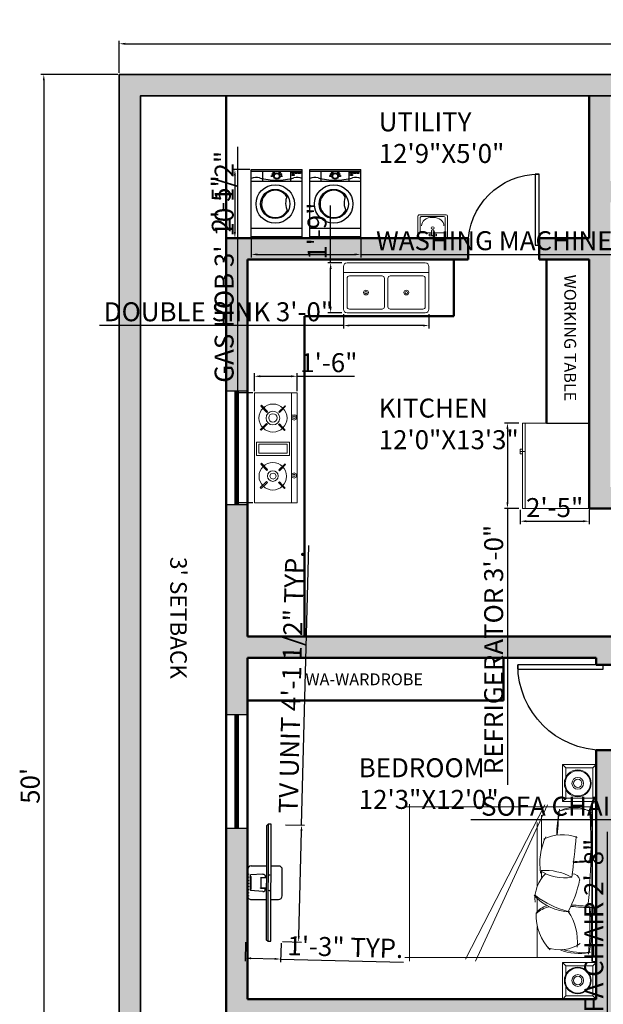
# Model space of a CAD drawing. Units: inches. Extents: x 2442 to 3851, y 589 to 2836.
# Tile 4 of 22: x 2452 to 2698, y 1610 to 2025. Entities that reach past the tile are written whole.
import ezdxf

# ---------------------------------------------------------------- set-up
doc = ezdxf.new("R2010")
doc.units = ezdxf.units.IN
for name, color, linetype, lineweight in [('0.10', 252, 'Continuous', 9), ('0.15', 34, 'Continuous', 15), ('A-ANNO-DIMS', 2, 'Continuous', 18), ('A-ANNO-TEXT', 7, 'Continuous', 18), ('A-AREA-IDEN', 7, 'Continuous', 18), ('A-DOOR', 4, 'Continuous', 25), ('A-EQPM', 9, 'Continuous', 18), ('A-FLOR-FIXT', 8, 'Continuous', 18), ('A-FURN', 8, 'Continuous', 18), ('A-GLAZ', 1, 'Continuous', 25), ('A-WALL', 7, 'Continuous', 50), ('A-WALL-PATT', 8, 'Continuous', 13), ('C-PROP', 7, 'Continuous', 35)]:
    doc.layers.add(name, color=color, linetype=linetype, lineweight=lineweight)
doc.layers.add('window', color=130, linetype='Continuous')
doc.layers.add('Сантехника', color=7, linetype='Continuous')
doc.styles.get("Standard").update_dxf_attribs({"font": 'arial.ttf'})
doc.dimstyles.new('ISO-25', dxfattribs={"dimtxt": 8, "dimasz": 2.5, "dimexe": 1.25, "dimexo": 0.625, "dimtad": 1, "dimlunit": 3, "dimtxsty": 'Standard', "dimcen": 2.5, "dimadec": 0, "dimazin": 0, "dimtfac": 1, "dimtmove": 0, "dimatfit": 3, "dimfxl": 1, "dimarcsym": 0})

# ---------------------------------------------------------------- blocks, each defined once
blk = doc.blocks.new('*U23')
for p, q in [((0, 0), (0, -6)), ((36, 0), (36, -6))]:
    blk.add_line(p, q)
blk.add_lwpolyline([(0, 0), (0, 36), (1.75, 36), (1.75, 0)], close=True)
blk.add_arc((0, 0), 36, 0, 90)
blk = doc.blocks.new('*U24')
for p, q in [((0, 0), (0, -6)), ((30, 0), (30, -6))]:
    blk.add_line(p, q)
blk.add_lwpolyline([(0, 0), (0, 30), (1.75, 30), (1.75, 0)], close=True)
blk.add_arc((0, 0), 30, 0, 90)
blk = doc.blocks.new('Refrigerator-2 door - 36 in top')
for p, q in [((0, -26.999999), (36, -26.999999)), ((11, -27.999999), (11, -28.999999)), ((11, -28.999999), (13, -28.999999)), ((12, -26.999999), (12, -28.999999)), ((13, -28.999999), (13, -27.999999))]:
    blk.add_line(p, q)
blk.add_lwpolyline([(0, -27.999999), (0, 0), (36, 0), (36, -27.999999)], close=True)
blk = doc.blocks.new('camita')
at = {"layer": '0.10'}
for p, q in [((-0.85, -0.045), (0.85, -0.045)), ((-0.805, -0.045), (-0.805, -2.048)), ((0.805, -0.045), (0.805, -2.048)), ((-0.827, -0.521), (0.846, -1.293)), ((-0.827, -0.548), (0.824, -1.399)), ((-0.716, -0.585), (-0.355, -0.585)), ((-0.638, -0.63), (0.043, -0.63)), ((-0.114, -0.585), (-0.049, -0.585)), ((0.175, -0.63), (0.318, -0.63)), ((0.474, -0.63), (0.805, -0.63)), ((-0.835, -2), (0.846, -2))]:
    blk.add_line(p, q, dxfattribs=at)
blk.add_lwpolyline([(-0.85, -0.041), (0.85, -0.041), (0.85, 0), (-0.85, 0)], close=True, dxfattribs=at)
for centre, radius, start, end in [((-0.457, -0.236), 0.344, 147.51, 213.8336), ((-0.2, -0.227), 0.586, 163.9263, 197.1409), ((-0.364, -5.846), 5.791, 83.8073, 94.1211), ((-0.51, -1.723), 1.678, 80.1255, 98.6619), ((2.353, -0.053), 2.58, 180.1063, 184.3854), ((-1.544, -0.245), 1.333, 359.9394, 7.5533), ((1.581, -0.289), 1.335, 170.3802, 178.9914), ((-1.44, -0.061), 1.712, 352.9291, 0.3959), ((0.452, -3.067), 3, 83.9026, 93.6759), ((0.486, -1.629), 1.578, 80.1602, 98.06), ((0.029, -0.138), 0.726, 342.5841, 6.0048), ((0.133, -0.17), 0.631, 339.923, 8.7433), ((-0.054, -0.363), 0.454, 159.3026, 206.5026), ((-0.007, -0.258), 0.0828, 100.018, 179.736), ((-0.293, -1.438), 1.29, 61.9749, 77.8435), ((0.627, -0.752), 0.551, 82.9691, 124.6739), ((0.32, -0.394), 0.404, 341.4524, 33.4512), ((-1.33, -9.675), 9.499, 82.2708, 84.9399), ((0.458, -0.545), 0.584, 151.0456, 184.1497), ((-0.534, -0.339), 0.487, 327.2644, 9.0473), ((-0.199, -0.274), 0.516, 310.7395, 359.0576), ((-0.567, -0.087), 0.906, 321.6953, 346.4626), ((-1.867, -14.986), 14.632, 84.6597, 85.7516), ((-0.46, 1.486), 1.909, 260.953, 268.6517), ((0.571, -0.432), 0.315, 192.9388, 221.9636), ((0.361, -0.133), 0.51, 267.2589, 315.2997), ((-0.2, 0.064), 0.667, 244.7809, 279.0606), ((0.179, -0.272), 0.383, 224.5284, 275.2229), ((0.438, -0.483), 0.19, 193.6849, 236.7035)]:
    blk.add_arc(centre, radius, start, end, dxfattribs=at)
blk = doc.blocks.new('VELADOR')
at = {"layer": '0.15'}
for p, q in [((-0.248, 0), (-0.203, -0.045)), ((0.248, 0), (0.202, -0.045)), ((-0.203, -0.405), (-0.248, -0.45)), ((0.248, -0.45), (0.202, -0.405))]:
    blk.add_line(p, q, dxfattribs=at)
blk.add_lwpolyline([(-0.248, 0), (-0.248, -0.45), (0.248, -0.45), (0.248, 0)], close=True, dxfattribs=at)
blk.add_lwpolyline([(0.092, -0.405), (0.202, -0.405), (0.202, -0.045), (-0.203, -0.045), (-0.203, -0.405), (-0.082, -0.405)], dxfattribs=at)
for radius in [0.18, 0.169, 0.0788, 0.0563]:
    blk.add_circle((0.005, -0.247), radius, dxfattribs=at)
blk = doc.blocks.new('Sink-double - 36 in top')
for p, q in [((-18, -4), (18, -4)), ((-0.75, -18.5), (-0.75, -6.5)), ((0.75, -6.5), (0.75, -18.5))]:
    blk.add_line(p, q)
for points in [[(-16.5, 0), (16.5, 0)], [(-18, -19.5), (-18, -1.5)], [(18, -1.5), (18, -19.5)], [(-16.5, -18.5), (-16.5, -6.5)], [(-15.5, -5.5), (-1.75, -5.5)], [(1.75, -5.5), (15.5, -5.5)], [(16.5, -6.5), (16.5, -18.5)], [(-1.75, -19.5), (-15.5, -19.5)], [(15.5, -19.5), (1.75, -19.5)], [(16.5, -21), (-16.5, -21)]]:
    blk.add_lwpolyline(points)
for centre, radius in [((-8.5, -12.5), 1), ((-8.5, -12.5), 0.5), ((8.5, -12.5), 1), ((8.5, -12.5), 0.5)]:
    blk.add_circle(centre, radius)
for centre, radius, start, end in [((-16.5, -1.5), 1.5, 90, 180), ((16.5, -1.5), 1.5, 0, 90), ((-15.5, -6.5), 1, 90, 180), ((-1.75, -6.5), 1, 0, 90), ((1.75, -6.5), 1, 90, 180), ((15.5, -6.5), 1, 0, 90), ((-16.5, -19.5), 1.5, 180, 270), ((-15.5, -18.5), 1, 180, 270), ((-1.75, -18.5), 1, 270, 0), ((1.75, -18.5), 1, 180, 270), ((15.5, -18.5), 1, 270, 0), ((16.5, -19.5), 1.5, 270, 0)]:
    blk.add_arc(centre, radius, start, end)
blk = doc.blocks.new('gas 1')
for points in [[(35.93, -1.87), (35.93, 0), (0, 0), (0, -1.87)], [(8.12, -0.94), (8.44, -1.56), (8.91, -1.87), (9.53, -1.56), (9.84, -0.94), (9.53, -0.31), (8.91, -0.16), (8.44, -0.31)], [(8.59, -0.94), (8.75, -1.25), (8.91, -1.41), (9.22, -1.25), (9.37, -0.94), (9.22, -0.78), (8.91, -0.62), (8.75, -0.78)], [(19.84, -13.28), (15.47, -13.28), (15.47, -2.5), (19.84, -2.5)], [(27.03, -0.94), (27.34, -1.56), (27.97, -1.87), (28.59, -1.56), (28.75, -0.94), (28.59, -0.31), (27.97, -0.16), (27.34, -0.31)], [(27.5, -0.94), (27.65, -1.25), (27.97, -1.41), (28.28, -1.25), (28.28, -0.94), (28.28, -0.62), (27.97, -0.62), (27.65, -0.62)], [(4.84, -3.91), (4.69, -4.06), (6.72, -6.09), (6.87, -5.78)], [(12.81, -3.91), (12.5, -3.75), (10.47, -5.78), (10.78, -5.94)], [(19.22, -12.5), (16.25, -12.5), (16.25, -3.28), (19.22, -3.28)], [(23.75, -3.91), (23.59, -4.06), (25.62, -6.09), (25.78, -5.78)], [(31.71, -3.91), (31.56, -3.75), (29.53, -5.78), (29.68, -5.94)], [(7.81, -7.81), (8.12, -8.59), (8.75, -8.91), (9.53, -8.59), (9.69, -7.81), (9.53, -7.19), (8.75, -6.87), (8.12, -7.19)], [(7.03, -10), (6.72, -9.69), (4.69, -11.72), (5, -12.03)], [(12.97, -11.56), (10.94, -9.69), (10.62, -9.84), (12.65, -11.87)], [(23.75, -11.72), (23.9, -12.03), (25.93, -10), (25.78, -9.69)], [(31.87, -11.56), (29.84, -9.69), (29.53, -9.84), (31.56, -11.87)]]:
    blk.add_lwpolyline(points, close=True)
blk.add_lwpolyline([(35.93, -1.87), (35.93, -13.9), (0, -13.9), (0, -1.87)])
for centre, radius in [((8.7, -7.92), 4.48), ((8.77, -7.89), 1.74), ((27.7, -7.86), 4.58), ((27.69, -7.89), 2.22), ((27.76, -7.89), 1.35)]:
    blk.add_circle(centre, radius)
blk = doc.blocks.new('TV')
at = {"color": 0}
for p, q in [((3967.27, 1784.85), (3967.05, 1784.65)), ((3967.76, 1763.68), (3967.54, 1763.86))]:
    blk.add_line(p, q, dxfattribs=at)
at = {"layer": 'window'}
for p, q in [((3967.54, 1763.86), (3967.05, 1784.65)), ((3964.41, 1777.23), (3967.22, 1777.3)), ((3968.01, 1777.32), (3969.36, 1777.35)), ((3966.53, 1775.82), (3964.33, 1775.61)), ((3964.34, 1775.34), (3964.45, 1775.34)), ((3964.34, 1775.31), (3964.43, 1775.32)), ((3966.14, 1775.2), (3967.01, 1775.22)), ((3966.14, 1775.18), (3967.27, 1775.2)), ((3966.14, 1775.18), (3966.14, 1775.2)), ((3966.3, 1773.29), (3966.26, 1775.18)), ((3966.19, 1773.28), (3967.31, 1773.31)), ((3966.19, 1773.26), (3967.05, 1773.28)), ((3966.19, 1773.26), (3966.19, 1773.28)), ((3964.39, 1773.06), (3964.48, 1773.06)), ((3964.39, 1773.04), (3964.5, 1773.04)), ((3966.61, 1772.66), (3964.4, 1772.77)), ((3964.55, 1771.15), (3967.36, 1771.22)), ((3968.15, 1771.24), (3969.5, 1771.27))]:
    blk.add_line(p, q, dxfattribs=at)
for points in [[(3968.33, 1763.69), (3967.83, 1784.86), (3967.27, 1784.85), (3967.76, 1763.68), (3968.33, 1763.69)], [(3963.86, 1771.81), (3963.75, 1776.54)], [(3964.4, 1772.77), (3964.33, 1775.61)], [(3964.48, 1773.06), (3964.43, 1775.32)], [(3964.5, 1773.04), (3964.45, 1775.34)], [(3970.16, 1771.96), (3970.05, 1776.69)]]:
    blk.add_lwpolyline(points, dxfattribs=at)
for points in [[(3966.53, 1775.82, -0.263666), (3966.93, 1775.69), (3967, 1775.57), (3967.01, 1775.22)], [(3966.61, 1772.66, 0.263666), (3967, 1772.81), (3967.06, 1772.93), (3967.05, 1773.28)]]:
    blk.add_lwpolyline(points, format="xyb", dxfattribs=at)
for centre, radius in [((3963.91, 1775.73), 0.0679), ((3963.93, 1775.17), 0.0679), ((3967.77, 1775.68), 0.0451), ((3963.94, 1774.6), 0.0679), ((3963.95, 1774.04), 0.0679), ((3963.97, 1773.48), 0.0679), ((3963.98, 1772.92), 0.0679), ((3963.99, 1772.35), 0.0679), ((3964.01, 1771.79), 0.0679), ((3967.83, 1772.86), 0.0451)]:
    blk.add_circle(centre, radius, dxfattribs=at)
for centre, start, end in [((3964.42, 1776.56), 91.3414, 181.3414), ((3969.38, 1776.67), 1.3414, 91.3414), ((3964.53, 1771.83), 181.3414, 271.3414), ((3969.49, 1771.94), 271.3414, 1.3414)]:
    blk.add_arc(centre, 0.676, start, end, dxfattribs=at)
blk = doc.blocks.new('wash')
at = {"layer": 'Сантехника'}
for p, q in [((4817.13, 2840.92), (4788.24, 2840.92)), ((4788.24, 2819.46), (4788.24, 2840.92)), ((4788.93, 2819.46), (4788.93, 2840.92)), ((4793.08, 2819.46), (4793.08, 2840.92)), ((4812.98, 2819.46), (4812.98, 2840.92)), ((4816.44, 2819.46), (4816.44, 2840.92)), ((4817.13, 2819.46), (4817.13, 2840.92)), ((4793.08, 2836.07), (4788.93, 2836.07)), ((4793.08, 2824.31), (4788.93, 2824.31)), ((4817.13, 2819.46), (4788.24, 2819.46)), ((4817.13, 2816.27), (4788.24, 2816.27)), ((4788.24, 2794.82), (4788.24, 2816.27)), ((4788.93, 2794.82), (4788.93, 2816.27)), ((4793.08, 2794.82), (4793.08, 2816.27)), ((4812.98, 2794.82), (4812.98, 2816.27)), ((4816.44, 2794.82), (4816.44, 2816.27)), ((4817.13, 2794.82), (4817.13, 2816.27)), ((4793.08, 2811.43), (4788.93, 2811.43)), ((4793.08, 2799.66), (4788.93, 2799.66)), ((4817.13, 2794.82), (4788.24, 2794.82))]:
    blk.add_line(p, q, dxfattribs=at)
for points in [[(4789.4, 2839.27), (4789.4, 2840.17), (4789.9, 2840.17), (4789.9, 2839.27)], [(4789.4, 2837.95), (4789.4, 2838.85), (4789.9, 2838.85), (4789.9, 2837.95)], [(4789.4, 2836.64), (4789.4, 2837.53), (4789.9, 2837.53), (4789.9, 2836.64)], [(4790.27, 2836.64), (4790.27, 2837.53), (4790.77, 2837.53), (4790.77, 2836.64)], [(4789.4, 2814.62), (4789.4, 2815.52), (4789.9, 2815.52), (4789.9, 2814.62)], [(4789.4, 2813.31), (4789.4, 2814.2), (4789.9, 2814.2), (4789.9, 2813.31)], [(4789.4, 2811.99), (4789.4, 2812.89), (4789.9, 2812.89), (4789.9, 2811.99)], [(4790.27, 2811.99), (4790.27, 2812.89), (4790.77, 2812.89), (4790.77, 2811.99)]]:
    blk.add_lwpolyline(points, close=True, dxfattribs=at)
for centre, radius in [((4802.77, 2829.54), 8.1), ((4802.77, 2829.54), 6.17), ((4789.46, 2831.45), 0.271), ((4790.19, 2831.93), 0.271), ((4790.98, 2832.18), 0.271), ((4789.46, 2828.92), 0.271), ((4790.98, 2830.19), 1.34), ((4790.98, 2830.19), 1.07), ((4790.19, 2828.4), 0.271), ((4790.98, 2828.15), 0.271), ((4802.77, 2804.9), 8.1), ((4802.77, 2804.9), 6.17), ((4789.46, 2806.8), 0.271), ((4790.98, 2805.55), 1.34), ((4790.19, 2807.28), 0.271), ((4790.98, 2807.53), 0.271), ((4789.46, 2804.27), 0.271), ((4790.98, 2805.55), 1.07), ((4790.19, 2803.75), 0.271), ((4790.98, 2803.5), 0.271)]:
    blk.add_circle(centre, radius, dxfattribs=at)
for centre, radius, start, end in [((4796.44, 2838.85), 4.89, 154.895, 196.6068), ((4762.87, 2829.66), 29.92, 1.0206, 15.0937), ((4802.77, 2829.54), 5.77, 121.8067, 62.1506), ((4802.39, 2840.74), 6.83, 243.19, 300.7673), ((4762.87, 2830.72), 29.92, 344.9063, 358.9794), ((4796.44, 2821.54), 4.89, 163.3932, 205.105), ((4796.44, 2814.2), 4.89, 154.895, 196.6068), ((4762.87, 2805.01), 29.92, 1.0206, 15.0937), ((4802.77, 2804.9), 5.77, 121.8067, 62.1506), ((4802.39, 2816.1), 6.83, 243.19, 300.7673), ((4762.87, 2806.08), 29.92, 344.9063, 358.9794), ((4796.44, 2796.89), 4.89, 163.3932, 205.105)]:
    blk.add_arc(centre, radius, start, end, dxfattribs=at)
blk = doc.blocks.new('Rac7')
at = {"color": 0}
for p, q in [((-39501, -24232), (-39501, -23830)), ((-39474, -23808), (-38988, -23808)), ((-39457, -23859), (-39457, -24115)), ((-39032, -23838), (-39430, -23838)), ((-39221, -23855), (-39241, -23855)), ((-39005, -24115), (-39005, -23859)), ((-39005, -23859), (-39005, -23859)), ((-38961, -23830), (-38961, -24232)), ((-38961, -24232), (-39501, -24232)), ((-39430, -24136), (-39253, -24136)), ((-39297, -24164), (-39253, -24164)), ((-39297, -24194), (-39297, -24164)), ((-39165, -24194), (-39297, -24194)), ((-39253, -24186), (-39253, -24094)), ((-39253, -24186), (-39209, -24186)), ((-39209, -24186), (-39209, -24094)), ((-39209, -24136), (-39032, -24136)), ((-39209, -24164), (-39165, -24164)), ((-39165, -24164), (-39165, -24194))]:
    blk.add_line(p, q, dxfattribs=at)
at = {"color": 0, "extrusion": (0, 0, -1)}
for centre, major_axis, start_param, end_param in [((-39474, -23830), (-27, 0), 0, 1.570796), ((-39430, -23859), (-27, 0), 0, 1.570796), ((-39241, -24007), (-194, 0), 0, 1.570796), ((-39221, -24007), (-194, 0), 1.570796, 3.141593), ((-39032, -23859), (-27, 0), 1.570796, 3.141593), ((-38988, -23830), (-27, 0), 1.570796, 3.141593), ((-39430, -24115), (-27, 0), -1.570796, 0), ((-39231, -24104), (-25.3, 0), 0.552816, 2.588777), ((-39032, -24115), (-27, 0), -3.141593, -1.570796)]:
    blk.add_ellipse(centre, major_axis=major_axis, ratio=0.785714, start_param=start_param, end_param=end_param, dxfattribs=at)
blk.add_ellipse((-39231, -24048), major_axis=(-27.9, 0), ratio=0.785714, dxfattribs=at)
blk = doc.blocks.new('*D31')
at = {"layer": 'A-ANNO-DIMS', "color": 0, "lineweight": -2, "transparency": 16777216}
for p, q in [((2493.6, 2002.49), (2493.6, 2016.02)), ((2496.1, 2014.77), (3091.1, 2014.77)), ((3093.6, 2002.49), (3093.6, 2016.02))]:
    blk.add_line(p, q, dxfattribs=at)
at = {"layer": 'A-ANNO-DIMS', "color": 0, "transparency": 16777216}
for points in [[(2496.1, 2015.19), (2496.1, 2014.36), (2493.6, 2014.77)], [(3091.1, 2015.19), (3091.1, 2014.36), (3093.6, 2014.77)]]:
    blk.add_solid(points, dxfattribs=at)
at = {"layer": 'Defpoints', "color": 0, "transparency": 16777216}
for p in [(3093.6, 2014.77), (2493.6, 2001.86), (3093.6, 2001.86)]:
    blk.add_point(p, dxfattribs=at)
at = {"layer": 'A-ANNO-DIMS', "color": 0, "transparency": 16777216, "insert": (2793.6, 2019.48), "char_height": 8, "attachment_point": 5}
blk.add_mtext("50'", dxfattribs=at)
blk = doc.blocks.new('*D32')
at = {"layer": 'A-ANNO-DIMS', "color": 0, "lineweight": -2, "transparency": 16777216}
for p, q in [((2492.97, 2001.86), (2460.53, 2001.86)), ((2461.78, 1999.36), (2461.78, 1404.36)), ((2492.97, 1401.86), (2460.53, 1401.86))]:
    blk.add_line(p, q, dxfattribs=at)
at = {"layer": 'A-ANNO-DIMS', "color": 0, "transparency": 16777216}
for points in [[(2461.36, 1999.36), (2462.2, 1999.36), (2461.78, 2001.86)], [(2461.36, 1404.36), (2462.2, 1404.36), (2461.78, 1401.86)]]:
    blk.add_solid(points, dxfattribs=at)
at = {"layer": 'Defpoints', "color": 0, "transparency": 16777216}
for p in [(2493.6, 2001.86), (2461.78, 1401.86), (2493.6, 1401.86)]:
    blk.add_point(p, dxfattribs=at)
at = {"layer": 'A-ANNO-DIMS', "color": 0, "transparency": 16777216, "insert": (2457.07, 1701.86), "char_height": 8, "attachment_point": 5, "rotation": 90}
blk.add_mtext("50'", dxfattribs=at)
blk = doc.blocks.new('*D146')
at = {"layer": 'A-ANNO-DIMS', "color": 0, "lineweight": -2, "transparency": 16777216}
for p, q in [((2570.43, 1685.32), (2573.43, 1803.21)), ((2563.67, 1685.49), (2571.68, 1685.29)), ((2569.24, 1638.53), (2570.37, 1682.82)), ((2562.41, 1636.21), (2570.43, 1636))]:
    blk.add_line(p, q, dxfattribs=at)
at = {"layer": 'A-ANNO-DIMS', "color": 0, "transparency": 16777216}
for points in [[(2569.95, 1682.83), (2570.79, 1682.81), (2570.43, 1685.32)], [(2568.83, 1638.54), (2569.66, 1638.52), (2569.18, 1636.04)]]:
    blk.add_solid(points, dxfattribs=at)
at = {"layer": 'Defpoints', "color": 0, "transparency": 16777216}
for p in [(2563.04, 1685.51), (2570.43, 1685.32), (2561.79, 1636.22)]:
    blk.add_point(p, dxfattribs=at)
at = {"layer": 'A-ANNO-DIMS', "color": 0, "transparency": 16777216, "insert": (2567.21, 1745.63), "char_height": 8, "attachment_point": 5, "rotation": 88.5431}
blk.add_mtext('TV UNIT 4\'-1 1/2" TYP.', dxfattribs=at)
blk = doc.blocks.new('*D147')
at = {"layer": 'A-ANNO-DIMS', "color": 0, "lineweight": -2, "transparency": 16777216}
for p, q in [((2546.82, 1635.98), (2546.62, 1627.96)), ((2561.77, 1635.6), (2561.57, 1627.58)), ((2549.15, 1629.15), (2559.1, 1628.89)), ((2561.6, 1628.83), (2613.34, 1627.51))]:
    blk.add_line(p, q, dxfattribs=at)
at = {"layer": 'A-ANNO-DIMS', "color": 0, "transparency": 16777216}
for points in [[(2549.16, 1629.56), (2549.14, 1628.73), (2546.65, 1629.21)], [(2559.11, 1629.31), (2559.09, 1628.48), (2561.6, 1628.83)]]:
    blk.add_solid(points, dxfattribs=at)
at = {"layer": 'Defpoints', "color": 0, "transparency": 16777216}
for p in [(2546.84, 1636.6), (2561.79, 1636.22), (2561.6, 1628.83)]:
    blk.add_point(p, dxfattribs=at)
at = {"layer": 'A-ANNO-DIMS', "color": 0, "transparency": 16777216, "insert": (2588.84, 1632.85), "char_height": 8, "attachment_point": 5, "rotation": 358.5431}
blk.add_mtext('1\'-3" TYP.', dxfattribs=at)
blk = doc.blocks.new('*D150')
at = {"layer": 'A-ANNO-DIMS', "color": 0, "lineweight": -2, "transparency": 16777216}
for p, q in [((2699.39, 1586.16), (2699.39, 1682.55)), ((2695.22, 1586.16), (2700.64, 1586.16)), ((2699.39, 1556.72), (2699.39, 1583.66)), ((2695.22, 1554.22), (2700.64, 1554.22))]:
    blk.add_line(p, q, dxfattribs=at)
at = {"layer": 'A-ANNO-DIMS', "color": 0, "transparency": 16777216}
for points in [[(2698.97, 1583.66), (2699.81, 1583.66), (2699.39, 1586.16)], [(2698.97, 1556.72), (2699.81, 1556.72), (2699.39, 1554.22)]]:
    blk.add_solid(points, dxfattribs=at)
at = {"layer": 'Defpoints', "color": 0, "transparency": 16777216}
for p in [(2694.6, 1586.16), (2699.39, 1586.16), (2694.6, 1554.22)]:
    blk.add_point(p, dxfattribs=at)
at = {"layer": 'A-ANNO-DIMS', "color": 0, "transparency": 16777216, "insert": (2694.63, 1635.61), "char_height": 8, "attachment_point": 5, "rotation": 90}
blk.add_mtext('SOFA CHAIR 2\'-8"', dxfattribs=at)
blk = doc.blocks.new('*D154')
at = {"layer": 'A-ANNO-DIMS', "color": 0, "lineweight": -2, "transparency": 16777216}
for p, q in [((2765.6, 1687.48), (2641.71, 1687.48)), ((2765.6, 1684.49), (2765.6, 1688.73)), ((2787.22, 1687.48), (2768.1, 1687.48)), ((2789.72, 1684.49), (2789.72, 1688.73))]:
    blk.add_line(p, q, dxfattribs=at)
at = {"layer": 'A-ANNO-DIMS', "color": 0, "transparency": 16777216}
for points in [[(2768.1, 1687.9), (2768.1, 1687.07), (2765.6, 1687.48)], [(2787.22, 1687.9), (2787.22, 1687.07), (2789.72, 1687.48)]]:
    blk.add_solid(points, dxfattribs=at)
at = {"layer": 'Defpoints', "color": 0, "transparency": 16777216}
for p in [(2765.6, 1687.48), (2765.6, 1683.86), (2789.72, 1683.86)]:
    blk.add_point(p, dxfattribs=at)
at = {"layer": 'A-ANNO-DIMS', "color": 0, "transparency": 16777216, "insert": (2702.4, 1692.25), "char_height": 8, "attachment_point": 5}
blk.add_mtext('SOFA CHAIR 2\'-0" TYP.', dxfattribs=at)
blk = doc.blocks.new('*D174')
at = {"layer": 'A-ANNO-DIMS', "color": 0, "lineweight": -2, "transparency": 16777216}
for p, q in [((2661.97, 1854.86), (2655.95, 1854.86)), ((2657.2, 1852.36), (2657.2, 1821.36)), ((2661.97, 1818.86), (2655.95, 1818.86)), ((2657.2, 1818.86), (2657.2, 1702.37))]:
    blk.add_line(p, q, dxfattribs=at)
at = {"layer": 'A-ANNO-DIMS', "color": 0, "transparency": 16777216}
for points in [[(2656.78, 1852.36), (2657.62, 1852.36), (2657.2, 1854.86)], [(2656.78, 1821.36), (2657.62, 1821.36), (2657.2, 1818.86)]]:
    blk.add_solid(points, dxfattribs=at)
at = {"layer": 'Defpoints', "color": 0, "transparency": 16777216}
for p in [(2662.6, 1854.86), (2657.2, 1818.86), (2662.6, 1818.86)]:
    blk.add_point(p, dxfattribs=at)
at = {"layer": 'A-ANNO-DIMS', "color": 0, "transparency": 16777216, "insert": (2652.43, 1759.37), "char_height": 8, "attachment_point": 5, "rotation": 90}
blk.add_mtext('REFRIGERATOR 3\'-0"', dxfattribs=at)
blk = doc.blocks.new('*D175')
at = {"layer": 'A-ANNO-DIMS', "color": 0, "lineweight": -2, "transparency": 16777216}
for p, q in [((2662.6, 1818.24), (2662.6, 1812.21)), ((2691.6, 1818.24), (2691.6, 1812.21)), ((2665.1, 1813.46), (2689.1, 1813.46))]:
    blk.add_line(p, q, dxfattribs=at)
at = {"layer": 'A-ANNO-DIMS', "color": 0, "transparency": 16777216}
for points in [[(2665.1, 1813.88), (2665.1, 1813.05), (2662.6, 1813.46)], [(2689.1, 1813.88), (2689.1, 1813.05), (2691.6, 1813.46)]]:
    blk.add_solid(points, dxfattribs=at)
at = {"layer": 'Defpoints', "color": 0, "transparency": 16777216}
for p in [(2662.6, 1818.86), (2691.6, 1818.86), (2691.6, 1813.46)]:
    blk.add_point(p, dxfattribs=at)
at = {"layer": 'A-ANNO-DIMS', "color": 0, "transparency": 16777216, "insert": (2677.1, 1818.17), "char_height": 8, "attachment_point": 5}
blk.add_mtext('2\'-5"', dxfattribs=at)
blk = doc.blocks.new('*D176')
at = {"layer": 'A-ANNO-DIMS', "color": 0, "lineweight": -2, "transparency": 16777216}
for p, q in [((2588.08, 1900.75), (2588.08, 1894.72)), ((2624.08, 1900.75), (2624.08, 1894.72)), ((2588.08, 1895.97), (2485.21, 1895.97)), ((2621.58, 1895.97), (2590.58, 1895.97))]:
    blk.add_line(p, q, dxfattribs=at)
at = {"layer": 'A-ANNO-DIMS', "color": 0, "transparency": 16777216}
for points in [[(2590.58, 1896.39), (2590.58, 1895.56), (2588.08, 1895.97)], [(2621.58, 1896.39), (2621.58, 1895.56), (2624.08, 1895.97)]]:
    blk.add_solid(points, dxfattribs=at)
at = {"layer": 'Defpoints', "color": 0, "transparency": 16777216}
for p in [(2588.08, 1901.37), (2624.08, 1901.37), (2588.08, 1895.97)]:
    blk.add_point(p, dxfattribs=at)
at = {"layer": 'A-ANNO-DIMS', "color": 0, "transparency": 16777216, "insert": (2535.39, 1900.74), "char_height": 8, "attachment_point": 5}
blk.add_mtext('DOUBLE SINK 3\'-0"', dxfattribs=at)
blk = doc.blocks.new('*D177')
at = {"layer": 'A-ANNO-DIMS', "color": 0, "lineweight": -2, "transparency": 16777216}
for p, q in [((2582.68, 1922.37), (2582.68, 1946.64)), ((2587.45, 1922.37), (2581.43, 1922.37)), ((2582.68, 1903.87), (2582.68, 1919.87)), ((2587.45, 1901.37), (2581.43, 1901.37))]:
    blk.add_line(p, q, dxfattribs=at)
at = {"layer": 'A-ANNO-DIMS', "color": 0, "transparency": 16777216}
for points in [[(2582.26, 1919.87), (2583.09, 1919.87), (2582.68, 1922.37)], [(2582.26, 1903.87), (2583.09, 1903.87), (2582.68, 1901.37)]]:
    blk.add_solid(points, dxfattribs=at)
at = {"layer": 'Defpoints', "color": 0, "transparency": 16777216}
for p in [(2582.68, 1922.37), (2588.08, 1922.37), (2588.08, 1901.37)]:
    blk.add_point(p, dxfattribs=at)
at = {"layer": 'A-ANNO-DIMS', "color": 0, "transparency": 16777216, "insert": (2577.97, 1935.76), "char_height": 8, "attachment_point": 5, "rotation": 90}
blk.add_mtext('1\'-9"', dxfattribs=at)
blk = doc.blocks.new('*D178')
at = {"layer": 'A-ANNO-DIMS', "color": 0, "lineweight": -2, "transparency": 16777216}
for p, q in [((2543.59, 1867.6), (2543.59, 1971.38)), ((2549.93, 1867.6), (2542.34, 1867.6)), ((2543.59, 1823.66), (2543.59, 1865.1)), ((2549.93, 1821.16), (2542.34, 1821.16))]:
    blk.add_line(p, q, dxfattribs=at)
at = {"layer": 'A-ANNO-DIMS', "color": 0, "transparency": 16777216}
for points in [[(2543.17, 1865.1), (2544.01, 1865.1), (2543.59, 1867.6)], [(2543.17, 1823.66), (2544.01, 1823.66), (2543.59, 1821.16)]]:
    blk.add_solid(points, dxfattribs=at)
at = {"layer": 'Defpoints', "color": 0, "transparency": 16777216}
for p in [(2543.59, 1867.6), (2550.56, 1867.6), (2550.56, 1821.16)]:
    blk.add_point(p, dxfattribs=at)
at = {"layer": 'A-ANNO-DIMS', "color": 0, "transparency": 16777216, "insert": (2538.82, 1920.74), "char_height": 8, "attachment_point": 5, "rotation": 90}
blk.add_mtext('GAS HOB 3\'-10 1/2"', dxfattribs=at)
blk = doc.blocks.new('*D179')
at = {"layer": 'A-ANNO-DIMS', "color": 0, "lineweight": -2, "transparency": 16777216}
for p, q in [((2550.56, 1868.23), (2550.56, 1875.82)), ((2553.06, 1874.57), (2566.03, 1874.57)), ((2568.53, 1868.23), (2568.53, 1875.82)), ((2568.53, 1874.57), (2592.79, 1874.57))]:
    blk.add_line(p, q, dxfattribs=at)
at = {"layer": 'A-ANNO-DIMS', "color": 0, "transparency": 16777216}
for points in [[(2553.06, 1874.99), (2553.06, 1874.16), (2550.56, 1874.57)], [(2566.03, 1874.99), (2566.03, 1874.16), (2568.53, 1874.57)]]:
    blk.add_solid(points, dxfattribs=at)
at = {"layer": 'Defpoints', "color": 0, "transparency": 16777216}
for p in [(2568.53, 1874.57), (2550.56, 1867.6), (2568.53, 1867.6)]:
    blk.add_point(p, dxfattribs=at)
at = {"layer": 'A-ANNO-DIMS', "color": 0, "transparency": 16777216, "insert": (2581.91, 1879.28), "char_height": 8, "attachment_point": 5}
blk.add_mtext('1\'-6"', dxfattribs=at)
blk = doc.blocks.new('*D180')
at = {"layer": 'A-ANNO-DIMS', "color": 0, "lineweight": -2, "transparency": 16777216}
for p, q in [((2549.24, 1932.24), (2549.24, 1924.7)), ((2595.34, 1932.24), (2595.34, 1924.7)), ((2551.74, 1925.95), (2592.84, 1925.95)), ((2595.34, 1925.95), (2738.05, 1925.95))]:
    blk.add_line(p, q, dxfattribs=at)
at = {"layer": 'A-ANNO-DIMS', "color": 0, "transparency": 16777216}
for points in [[(2551.74, 1926.37), (2551.74, 1925.53), (2549.24, 1925.95)], [(2592.84, 1926.37), (2592.84, 1925.53), (2595.34, 1925.95)]]:
    blk.add_solid(points, dxfattribs=at)
at = {"layer": 'Defpoints', "color": 0, "transparency": 16777216}
for p in [(2549.24, 1932.86), (2595.34, 1932.86), (2595.34, 1925.95)]:
    blk.add_point(p, dxfattribs=at)
at = {"layer": 'A-ANNO-DIMS', "color": 0, "transparency": 16777216, "insert": (2667.94, 1930.71), "char_height": 8, "attachment_point": 5}
blk.add_mtext('WASHING MACHINE 3\'-10"', dxfattribs=at)
blk = doc.blocks.new('*D181')
at = {"layer": 'A-ANNO-DIMS', "color": 0, "lineweight": -2, "transparency": 16777216}
for p, q in [((2548.62, 1961.76), (2541.08, 1961.76)), ((2542.33, 1959.26), (2542.33, 1935.36)), ((2548.62, 1932.86), (2541.08, 1932.86))]:
    blk.add_line(p, q, dxfattribs=at)
at = {"layer": 'A-ANNO-DIMS', "color": 0, "transparency": 16777216}
for points in [[(2541.91, 1959.26), (2542.74, 1959.26), (2542.33, 1961.76)], [(2541.91, 1935.36), (2542.74, 1935.36), (2542.33, 1932.86)]]:
    blk.add_solid(points, dxfattribs=at)
at = {"layer": 'Defpoints', "color": 0, "transparency": 16777216}
for p in [(2549.24, 1961.76), (2542.33, 1932.86), (2549.24, 1932.86)]:
    blk.add_point(p, dxfattribs=at)
at = {"layer": 'A-ANNO-DIMS', "color": 0, "transparency": 16777216, "insert": (2537.62, 1947.31), "char_height": 8, "attachment_point": 5, "rotation": 90}
blk.add_mtext('2\'-5"', dxfattribs=at)

msp = doc.modelspace()

# ---------------------------------------------------------------- hatches: boundary and pattern name
at = {"layer": 'A-WALL-PATT'}
h = msp.add_hatch(color=256, dxfattribs=at)
h.dxf.hatch_style = 1
h.paths.add_polyline_path([(2502.599, 1992.864), (2719.571, 1992.864), (2719.687, 1994.649), (2720.167, 1997.319), (2721.479, 1992.864), (2726.325, 1992.864), (2727.448, 1994.93), (2729.005, 1997.153), (2728.372, 1992.864), (2728.871, 1992.864), (2730.114, 1994.505), (2731.833, 1996.09), (2730.966, 1993.206), (2730.864, 1992.864), (2771.772, 1992.864), (2771.887, 1994.649), (2772.368, 1997.319), (2773.68, 1992.864), (2778.526, 1992.864), (2779.649, 1994.93), (2781.206, 1997.153), (2780.572, 1992.864), (2781.072, 1992.864), (2782.315, 1994.505), (2784.034, 1996.09), (2783.167, 1993.206), (2783.065, 1992.864), (2821.282, 1992.864), (2821.398, 1994.649), (2821.878, 1997.319), (2823.19, 1992.864), (2828.036, 1992.864), (2829.159, 1994.93), (2830.716, 1997.153), (2830.083, 1992.864), (2830.582, 1992.864), (2831.825, 1994.505), (2833.544, 1996.09), (2832.677, 1993.206), (2832.575, 1992.864), (2869.287, 1992.864), (2869.403, 1994.649), (2869.884, 1997.319), (2871.195, 1992.864), (2876.042, 1992.864), (2877.165, 1994.93), (2878.721, 1997.153), (2878.088, 1992.864), (2878.587, 1992.864), (2879.83, 1994.505), (2881.55, 1996.09), (2880.682, 1993.206), (2880.58, 1992.864), (2919.335, 1992.864), (2919.451, 1994.649), (2919.932, 1997.319), (2921.243, 1992.864), (2926.09, 1992.864), (2927.213, 1994.93), (2928.77, 1997.153), (2928.136, 1992.864), (2928.635, 1992.864), (2929.878, 1994.505), (2931.598, 1996.09), (2930.73, 1993.206), (2930.628, 1992.864), (2966.155, 1992.864), (2966.27, 1994.649), (2966.751, 1997.319), (2968.063, 1992.864), (2972.909, 1992.864), (2974.032, 1994.93), (2975.589, 1997.153), (2974.955, 1992.864), (2975.455, 1992.864), (2976.698, 1994.505), (2978.417, 1996.09), (2977.55, 1993.206), (2977.448, 1992.864), (3010.53, 1992.864), (3010.646, 1994.649), (3011.127, 1997.319), (3012.438, 1992.864), (3017.285, 1992.864), (3018.408, 1994.93), (3019.964, 1997.153), (3019.331, 1992.864), (3019.83, 1992.864), (3021.073, 1994.505), (3022.793, 1996.09), (3021.925, 1993.206), (3021.823, 1992.864), (3057.996, 1992.864), (3058.45, 1995.382), (3059.191, 1992.864), (3065.64, 1992.864), (3067.287, 1995.216), (3066.94, 1992.864), (3068.717, 1992.864), (3070.116, 1994.153), (3069.728, 1992.864), (3084.599, 1992.864), (3084.599, 1983.791), (3085.291, 1983.828), (3084.599, 1983.434), (3084.599, 1932.114), (3085.291, 1932.151), (3084.599, 1931.757), (3084.599, 1886.278), (3085.291, 1886.315), (3084.599, 1885.921), (3084.599, 1410.864), (3066.599, 1410.864), (3066.599, 1401.864), (3093.599, 1401.864), (3093.599, 2001.864), (2493.599, 2001.864), (2493.599, 1401.864), (2538.599, 1401.864), (2538.599, 1410.864), (2502.599, 1410.864)])
h.paths.add_polyline_path([(2738.599, 1410.864), (2547.599, 1410.864), (2547.599, 1401.864), (2738.599, 1401.864)], flags=17)
h.paths.add_polyline_path([(2910.599, 1410.864), (2792.599, 1410.864), (2792.599, 1401.864), (2910.599, 1401.864), (2910.599, 1402.864)], flags=17)
h = msp.add_hatch(color=256, dxfattribs=at)
h.dxf.hatch_style = 1
h.paths.add_polyline_path([(2799.599, 1467.864), (2775.599, 1467.864), (2775.599, 1458.864), (2799.599, 1458.864)])
h.paths.add_polyline_path([(2703.599, 1506.864), (2670.599, 1506.864), (2670.599, 1497.864), (2694.599, 1497.864), (2694.599, 1458.864), (2733.599, 1458.864), (2733.599, 1467.864), (2709.417, 1467.864), (2703.599, 1467.864)])
h.paths.add_polyline_path([(2604.599, 1506.864), (2593.599, 1506.864), (2593.599, 1497.864), (2604.599, 1497.864)])
h.paths.add_polyline_path([(2547.599, 1497.864), (2553.599, 1497.864), (2553.599, 1506.864), (2547.599, 1506.864), (2547.599, 1530.864), (2538.599, 1530.864), (2538.599, 1401.864), (2547.599, 1401.864)])
h.paths.add_polyline_path([(2547.599, 1683.864), (2538.599, 1683.864), (2538.599, 1578.864), (2547.599, 1578.864), (2547.599, 1602.864), (2694.599, 1602.864), (2694.599, 1554.864), (2703.599, 1554.864), (2703.599, 1716.864), (2694.599, 1716.864), (2694.599, 1611.864), (2547.599, 1611.864)])
h.paths.add_polyline_path([(2892.599, 1497.864), (2883.599, 1497.864), (2883.599, 1488.228), (2883.599, 1467.864), (2865.599, 1467.864), (2865.599, 1458.864), (2892.599, 1458.864)])
h.paths.add_polyline_path([(3048.599, 1722.864), (3039.599, 1722.864), (3039.599, 1716.864), (2937.599, 1716.864), (2937.599, 1710.864), (3039.599, 1710.864), (3039.599, 1685.364), (3048.599, 1685.364)])
h.paths.add_polyline_path([(3048.599, 1779.864), (3039.599, 1779.864), (3039.599, 1773.864), (2961.599, 1773.864), (2961.599, 1791.864), (2955.599, 1791.864), (2955.599, 1773.864), (2895.599, 1773.864), (2895.599, 1821.864), (2916.599, 1821.864), (2916.599, 1827.864), (2889.599, 1827.864), (2889.599, 1773.864), (2886.599, 1773.864), (2886.599, 1764.864), (2937.599, 1764.864), (2937.599, 1746.864), (2943.599, 1746.864), (2943.599, 1764.864), (2956.06, 1764.864), (3039.599, 1764.864), (3039.599, 1758.864), (3048.599, 1758.864)])
h.paths.add_polyline_path([(3048.599, 1827.864), (2976.475, 1827.864, -0.1284593), (2975.705, 1827.665), (2964.694, 1827.687, -0.1198794), (2963.972, 1827.864), (2946.599, 1827.864), (2946.599, 1821.864), (3039.599, 1821.864), (3039.599, 1815.864), (3048.599, 1815.864)])
h.paths.add_polyline_path([(3048.599, 1956.864), (3023.366, 1956.864), (3023.277, 1956.402), (3023.088, 1956.864), (3019.494, 1956.864), (3019.543, 1955.479), (3019.146, 1956.864), (3015.599, 1956.864), (3015.599, 1947.864), (3039.599, 1947.864), (3039.599, 1875.864), (3048.599, 1875.864), (3048.599, 1880.743), (3047.576, 1881.614), (3046.081, 1883.417), (3044.931, 1885.453), (3047.541, 1883.949), (3048.599, 1883.343), (3048.599, 1910.588), (3047.049, 1909.235), (3047.896, 1910.862), (3048.599, 1911.909), (3048.599, 1918.826), (3042.477, 1917.032), (3043.928, 1918.154), (3045.59, 1919.165), (3047.525, 1920.009), (3048.599, 1920.305), (3048.599, 1926.579), (3047.576, 1927.45), (3046.081, 1929.252), (3044.931, 1931.289), (3047.541, 1929.785), (3048.599, 1929.179)])
h.paths.add_polyline_path([(2967.599, 1956.864), (2932.171, 1956.864), (2932.082, 1956.402), (2931.893, 1956.864), (2928.299, 1956.864), (2928.348, 1955.479), (2927.951, 1956.864), (2898.599, 1956.864), (2898.599, 1947.864), (2967.599, 1947.864)])
h.paths.add_polyline_path([(2850.599, 1956.864), (2834.118, 1956.864), (2834.029, 1956.402), (2833.84, 1956.864), (2830.245, 1956.864), (2830.294, 1955.479), (2829.897, 1956.864), (2796.599, 1956.864), (2796.599, 1947.864), (2799.599, 1947.864), (2838.599, 1947.864), (2838.599, 1827.864), (2835.599, 1827.864), (2835.599, 1824.864), (2835.599, 1818.864), (2838.599, 1818.864), (2838.599, 1764.864), (2850.599, 1764.864), (2850.599, 1770.864), (2850.599, 1773.864), (2847.599, 1773.864), (2847.599, 1947.864), (2850.599, 1947.864)])
h.paths.add_polyline_path([(2700.599, 1947.864), (2730.599, 1947.864), (2730.599, 1956.864), (2700.599, 1956.864), (2700.599, 1992.864), (2691.599, 1992.864), (2691.599, 1932.864), (2670.599, 1932.864), (2670.599, 1923.864), (2691.599, 1923.864), (2691.599, 1818.864), (2799.599, 1818.864), (2799.599, 1827.864), (2700.599, 1827.864)])
h.paths.add_polyline_path([(2640.599, 1932.864), (2538.599, 1932.864), (2538.599, 1868.364), (2547.599, 1868.364), (2547.599, 1923.864), (2640.599, 1923.864), (2640.599, 1929.864)])
h.paths.add_polyline_path([(2547.599, 1820.364), (2538.599, 1820.364), (2538.599, 1731.864), (2547.599, 1731.864), (2547.599, 1755.864), (2694.599, 1755.864), (2694.599, 1752.864), (2697.599, 1752.864), (2703.599, 1752.864), (2703.599, 1764.864), (2547.599, 1764.864)])
h.paths.add_polyline_path([(2725.858, 1838.187), (2790.115, 1838.187), (2790.115, 1868.602), (2725.858, 1868.602)], flags=25)
h.paths.add_polyline_path([(2892.599, 1671.864), (2883.599, 1671.864), (2883.599, 1563.864), (2892.599, 1563.864), (2892.599, 1602.864), (3048.599, 1602.864), (3048.599, 1637.364), (3039.599, 1637.364), (3039.599, 1611.864), (2892.599, 1611.864)])

# ---------------------------------------------------------------- linework, layer by layer
at = {"layer": 'A-GLAZ'}
for p, q in [((2547.599, 1868.364), (2538.599, 1868.364)), ((2673.599, 1854.864), (2691.599, 1854.864)), ((2547.599, 1820.364), (2538.599, 1820.364)), ((2547.599, 1731.864), (2538.599, 1731.864)), ((2547.599, 1683.864), (2538.599, 1683.864))]:
    msp.add_line(p, q, dxfattribs=at)
at = {"layer": 'A-WALL'}
for p, q in [((2538.599, 1992.864), (2538.599, 1401.864)), ((2691.599, 1932.864), (2691.599, 1992.864)), ((2538.599, 1932.864), (2640.599, 1932.864)), ((2640.599, 1923.864), (2640.599, 1932.864)), ((2670.599, 1923.864), (2670.599, 1932.864)), ((2670.599, 1932.864), (2691.599, 1932.864)), ((2547.599, 1923.864), (2640.599, 1923.864)), ((2547.599, 1923.864), (2547.599, 1764.864)), ((2634.599, 1899.864), (2634.599, 1923.864)), ((2670.599, 1923.864), (2691.599, 1923.864)), ((2673.599, 1854.864), (2673.599, 1923.864)), ((2691.599, 1818.864), (2691.599, 1923.864)), ((2571.599, 1899.864), (2571.599, 1764.864)), ((2571.599, 1899.864), (2634.599, 1899.864)), ((2542.599, 1868.364), (2542.599, 1820.364)), ((2543.599, 1868.364), (2543.599, 1820.364)), ((2691.599, 1818.864), (2799.599, 1818.864)), ((2547.599, 1764.864), (2703.599, 1764.864)), ((2547.599, 1755.864), (2694.599, 1755.864)), ((2547.599, 1755.864), (2547.599, 1611.864)), ((2655.599, 1755.864), (2655.599, 1737.864)), ((2694.599, 1752.864), (2694.599, 1755.864)), ((2694.599, 1752.864), (2703.599, 1752.864)), ((2547.599, 1737.864), (2655.599, 1737.864)), ((2542.599, 1731.864), (2542.599, 1683.864)), ((2543.599, 1731.864), (2543.599, 1683.864)), ((2694.599, 1611.864), (2694.599, 1716.864)), ((2694.599, 1716.864), (2703.599, 1716.864)), ((2547.599, 1611.864), (2694.599, 1611.864))]:
    msp.add_line(p, q, dxfattribs=at)
at = {"layer": 'C-PROP'}
for points in [[(3066.599, 1401.864), (3093.599, 1401.864), (3093.599, 2001.864), (2493.599, 2001.864), (2493.599, 1401.864), (2738.599, 1401.864)], [(3066.599, 1410.864), (3084.599, 1410.864), (3084.599, 1992.864), (2502.599, 1992.864), (2502.599, 1410.864), (2538.599, 1410.864)]]:
    msp.add_lwpolyline(points, dxfattribs=at)

# ---------------------------------------------------------------- block references
at = {"layer": 'A-DOOR', "xscale": -1}
msp.add_blockref('*U24', (2670.599, 1929.864), dxfattribs=at)
at = {"layer": 'A-DOOR', "xscale": -1, "rotation": 90}
msp.add_blockref('*U23', (2697.599, 1752.864), dxfattribs=at)
at = {"layer": 'A-EQPM', "xscale": -1.292580420916565, "yscale": 1.292580420916565, "zscale": 1.292580420916565, "rotation": 270}
msp.add_blockref('gas 1', (2568.529, 1821.158), dxfattribs=at)
at = {"layer": 'A-EQPM', "rotation": 270}
msp.add_blockref('Refrigerator-2 door - 36 in top', (2691.599, 1854.864), dxfattribs=at)
at = {"layer": 'A-FLOR-FIXT', "rotation": 270}
msp.add_blockref('wash', (-245.575, 6749.997), dxfattribs=at)
at = {"layer": 'A-FLOR-FIXT', "xscale": -0.0231094998546128, "yscale": 0.0231094998546128, "zscale": 0.0231094998546128}
msp.add_blockref('Rac7', (1719.094, 2492.856), dxfattribs=at)
at = {"layer": 'A-FLOR-FIXT', "xscale": -1}
msp.add_blockref('Sink-double - 36 in top', (2606.078, 1922.374), dxfattribs=at)
at = {"layer": 'A-FURN'}
for name, p, xscale, yscale, zscale, rotation in [('VELADOR', (2694.599, 1703.089), 31.41542173157097, 31.41542173157097, 31.41542173157097, 270), ('camita', (2694.599, 1661.257), 39.375, 39.375, 39.375, 270), ('TV', (-6779.432, -2232.164), 2.327319231123021, 2.327319231123021, 2.327319231123021, 358.5430845181613), ('VELADOR', (2694.599, 1619.639), -31.41542173157097, 31.41542173157097, 31.41542173157097, 269.9999999999999)]:
    msp.add_blockref(name, p, dxfattribs=dict(at, xscale=xscale, yscale=yscale, zscale=zscale, rotation=rotation))

# ---------------------------------------------------------------- texts
at = {"layer": 'A-ANNO-TEXT', "attachment_point": 1, "rotation": 270}
for s, width, insert, char_height in [('{\\fTimes New Roman|b0|i0|c0|p18;WORKING TABLE}', 110.76054, (2686.144, 1917.453), 5), ("{\\fTimes New Roman|b0|i0|c0|p18;3' SETBACK}", 79.56037, (2522.055, 1798.403), 7)]:
    msp.add_mtext_dynamic_manual_height_columns(s, width=width, gutter_width=12.5, heights=[0], dxfattribs=dict(at, insert=insert, char_height=char_height))
at = {"layer": 'A-ANNO-TEXT', "insert": (2572.046, 1749.3), "char_height": 5, "attachment_point": 1}
msp.add_mtext_dynamic_manual_height_columns('{\\fTimes New Roman|b0|i0|c0|p18;WA-WARDROBE}', width=110.76054, gutter_width=12.5, heights=[0], dxfattribs=at)
at = {"layer": 'A-AREA-IDEN', "char_height": 8, "attachment_point": 1}
for s, insert in [('{\\fTimes New Roman|b0|i0|c0|p18;UTILITY\\P12\'9"X5\'0"}', (2602.937, 1985.863)), ('{\\fTimes New Roman|b0|i0|c0|p18;KITCHEN\\P12\'0"X13\'3"}', (2602.937, 1865.16)), ('{\\fTimes New Roman|b0|i0|c0|p18;BEDROOM\\P12\'3"X12\'0"}', (2594.523, 1713.494))]:
    msp.add_mtext_dynamic_manual_height_columns(s, width=110.76054, gutter_width=12.5, heights=[0], dxfattribs=dict(at, insert=insert))

# ---------------------------------------------------------------- dimensions: what is measured, and where the dimension line sits
at = {"layer": 'A-ANNO-DIMS'}
for base, p1, p2, override, picture, middle in [((3093.599, 2014.775), (2493.599, 2001.864), (3093.599, 2001.864), {"dimclrd": 0, "dimclre": 0, "dimclrt": 0}, '*D31', (2793.599, 2019.485)), ((2568.529, 1874.572), (2550.556, 1867.605), (2568.529, 1867.605), {"dimdec": 1, "dimrnd": 0, "dimzin": 1, "dimlunit": 4, "dimfrac": 2}, '*D179', (2581.91, 1879.282)), ((2691.599, 1813.464), (2662.599, 1818.864), (2691.599, 1818.864), {"dimdec": 1, "dimrnd": 0, "dimzin": 1, "dimlunit": 4, "dimfrac": 2}, '*D175', (2677.099, 1818.174))]:
    dim = msp.add_linear_dim(base=base, p1=p1, p2=p2, dimstyle='ISO-25', override=override, dxfattribs=at)
    dim.commit()
    dim.dimension.update_dxf_attribs({"geometry": picture, "text_midpoint": middle})
for base, p1, p2, angle, override, picture, middle in [((2461.781, 1401.864), (2493.599, 2001.864), (2493.599, 1401.864), 90, {"dimclrd": 0, "dimclre": 0, "dimclrt": 0}, '*D32', (2457.071, 1701.864)), ((2542.328, 1932.864), (2549.243, 1961.758), (2549.243, 1932.864), 270, {"dimdec": 1, "dimrnd": 0, "dimzin": 1, "dimlunit": 4, "dimfrac": 2}, '*D181', (2537.618, 1947.311)), ((2582.678, 1922.374), (2588.078, 1901.374), (2588.078, 1922.374), 90, {"dimdec": 1, "dimrnd": 0, "dimzin": 1, "dimlunit": 4, "dimfrac": 2}, '*D177', (2577.968, 1935.756))]:
    dim = msp.add_linear_dim(base=base, p1=p1, p2=p2, angle=angle, dimstyle='ISO-25', override=override, dxfattribs=at)
    dim.commit()
    dim.dimension.update_dxf_attribs({"geometry": picture, "text_midpoint": middle})
for base, p1, p2, angle, text, picture, middle in [((2543.589, 1867.605), (2550.556, 1821.158), (2550.556, 1867.605), 90, 'GAS HOB <>', '*D178', (2538.822, 1920.741)), ((2588.078, 1895.974), (2624.078, 1901.374), (2588.078, 1901.374), 180, 'DOUBLE SINK <>', '*D176', (2535.392, 1900.741)), ((2657.199, 1818.864), (2662.599, 1854.864), (2662.599, 1818.864), 270, 'REFRIGERATOR <>', '*D174', (2652.432, 1759.365)), ((2570.435, 1685.322), (2561.788, 1636.223), (2563.042, 1685.51), 88.54308, 'TV UNIT <> TYP.', '*D146', (2567.206, 1745.635)), ((2765.598, 1687.482), (2789.72, 1683.864), (2765.598, 1683.864), 180, 'SOFA CHAIR <> TYP.', '*D154', (2702.404, 1692.247)), ((2699.39, 1586.162), (2694.599, 1554.22), (2694.599, 1586.162), 90, 'SOFA CHAIR <>', '*D150', (2694.626, 1635.606)), ((2561.6, 1628.83), (2546.839, 1636.603), (2561.788, 1636.223), 358.54308, '<> TYP.', '*D147', (2588.842, 1632.851))]:
    dim = msp.add_linear_dim(base=base, p1=p1, p2=p2, angle=angle, text=text, dimstyle='ISO-25', override={"dimdec": 1, "dimrnd": 0, "dimzin": 1, "dimlunit": 4, "dimfrac": 2}, dxfattribs=at)
    dim.commit()
    dim.dimension.update_dxf_attribs({"geometry": picture, "text_midpoint": middle})
dim = msp.add_linear_dim(base=(2595.344, 1925.949), p1=(2549.243, 1932.864), p2=(2595.344, 1932.864), text='WASHING MACHINE <>', dimstyle='ISO-25', override={"dimdec": 1, "dimrnd": 0, "dimzin": 1, "dimlunit": 4, "dimfrac": 2}, dxfattribs=at)
dim.commit()
dim.dimension.update_dxf_attribs({"geometry": '*D180', "text_midpoint": (2667.945, 1930.713)})

doc.saveas('drawing.dxf')
